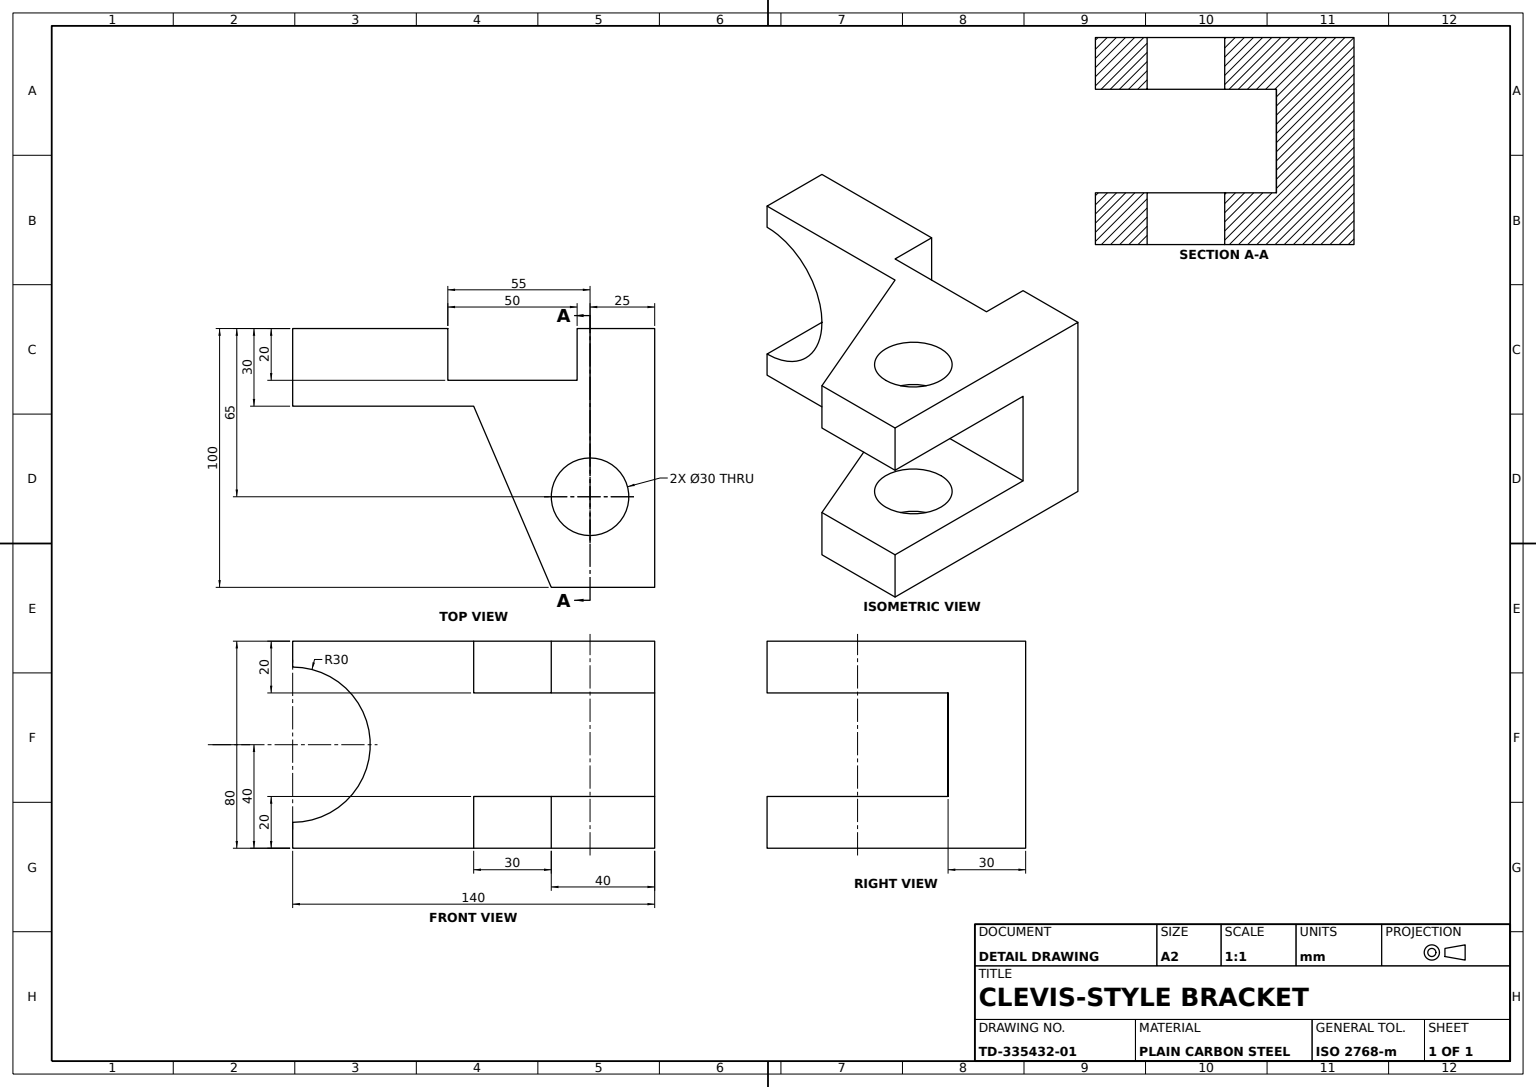
SolidWorks part; units mm, degrees
material "Plain Carbon Steel"
ref_plane "Front Plane" through (0, 0, 0) normal (0, 0, 1) x (1, 0, 0)
ref_plane "Top Plane" through (0, 0, 0) normal (0, 1, 0) x (1, 0, 0)
ref_plane "Right Plane" through (0, 0, 0) normal (1, 0, 0) x (0, 0, -1)
sketch "Base Profile Sketch" plane through (0, 0, 0) normal (0, 0, 1) x (1, 0, 0)
  line L0 (0, 0) -> (0, -80)
  line L1 (0, -80) -> (140, -80)
  line L2 (140, -80) -> (140, 0)
  line L3 (140, 0) -> (0, 0)
  arc A0 (0, -70) -> (0, -10) centre (0, -40) ccw
  dimension "D1" = 30
  dimension "D2" = 140
  dimension "D3" = 40
extrude "Base Block" add sketch "Base Profile Sketch" along normal blind 30 contours A0 L0 L1 L2 L3
sketch "Side Boss Sketch" plane through (0, -80, 0) normal (0, -1, 0) x (1, 0, 0)
  line L0 (140, 30) -> (140, 100)
  line L1 (140, 100) -> (100, 100)
  line L2 (140, 30) -> (70, 30)
  line L3 (140, 30) -> (140, 0) construction
  line L4 (0, 30) -> (140, 30) construction
  line L5 (70, 30) -> (100, 100)
  dimension "D1" = 40
extrude "Side Boss" add sketch "Side Boss Sketch" against normal blind 20
sketch "Top Boss Sketch" plane through (0, 0, 0) normal (0, 1, 0) x (1, 0, 0)
  line L0 (140, -30) -> (140, -100)
  line L1 (140, -100) -> (100, -100)
  line L2 (100, -100) -> (70, -30)
  line L3 (140, -30) -> (0, -30) construction
  line L4 (70, -30) -> (140, -30)
extrude "Top Boss" add sketch "Top Boss Sketch" against normal blind 20
sketch "Through Hole Sketch" plane through (0, -80, 0) normal (0, -1, 0) x (1, 0, 0)
  line L0 (140, 100) -> (140, 0) construction
  line L1 (0, 0) -> (140, 0) construction
  circle A0 centre (115, 65) radius 15
  dimension "D1" = 30
  dimension "D2" = 25
  dimension "D3" = 65
extrude "Coaxial Through Hole" cut sketch "Through Hole Sketch" against normal blind 80
sketch "Curved Relief Sketch" plane through (0, -80, 0) normal (0, -1, 0) x (1, 0, 0)
  line L0 (140, 100) -> (140, 0) construction
  line L1 (0, 0) -> (140, 0) construction
  line L2 (110, 0) -> (110, 20)
  line L3 (110, 20) -> (60, 20)
  line L4 (60, 20) -> (60, 0)
  line L5 (60, 0) -> (110, 0)
  dimension "D1" = 30
  dimension "D2" = 80
  dimension "D3" = 20
extrude "Curved Relief Cut" cut sketch "Curved Relief Sketch" against normal blind 80
